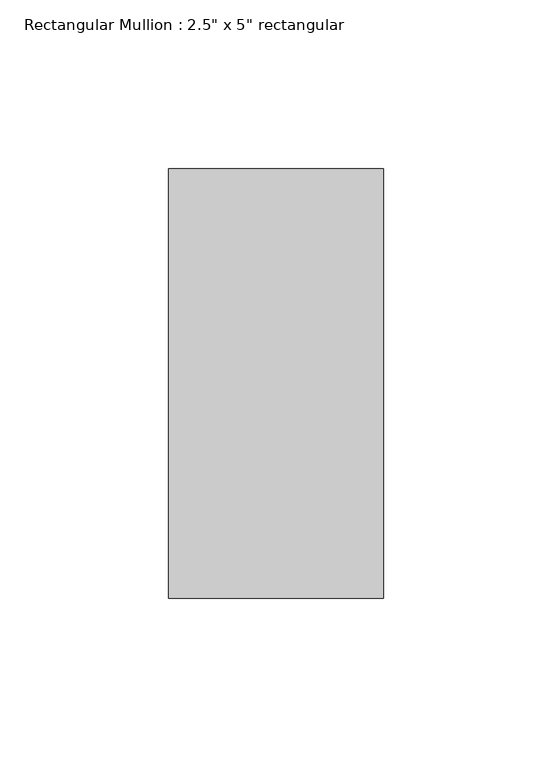
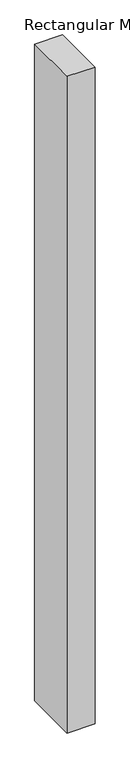
"""IFC4 building model written with IfcOpenShell, lengths in millimetres: member geometry."""

from ifc_helpers import new_model, si_unit, frame, origin, place, context, project, spatial, polyline, outline, extrude, source, transform, mapped, element, save


def member_acc0cca9(model_context):
    return source(origin(), model_context, "Body", "SweptSolid", [
        extrude(outline(polyline([(0.0, 63.5), (0.0, -63.5), (-63.5, -63.5), (-63.5, 63.5), (0.0, 63.5)])), frame((0.0, 0.0, -1570.4687519), z_axis=(0.0, 0.0, 1.0), x_axis=(1.0, 0.0, 0.0)), (0.0, 0.0, 1.0), 1570.4687519),
    ])


if __name__ == "__main__":
    model = new_model("IFC4")
    model_context = context("Model", 3, world=origin())
    ifc_project = project(units=[si_unit("LENGTHUNIT", "METRE", prefix="MILLI")], contexts=[model_context])
    site = spatial("IfcSite", under=ifc_project)
    building = spatial("IfcBuilding", under=site)
    placement = place(None, origin())
    member_shape = member_acc0cca9(model_context)
    element("IfcMember", 1, ObjectType="Rectangular Mullion : 2.5\" x 5\" rectangular", at=placement, inside=building, context=model_context, shape_type="MappedRepresentation", body=[
        mapped(member_shape, transform((0.0, 0.0, 0.0), x_axis=(1.0, 0.0, 0.0), y_axis=(0.0, 1.0, 0.0), z_axis=(0.0, 0.0, 1.0))),
    ])
    save(model, "model.ifc")

# Revit data of these elements
# Type "Rectangular Mullion : 2.5\" x 5\" rectangular"
#   built-in parameter 1007304 = 0.416667 (stored number, unit not read)
#   built-in parameter 1007301 = 0.104167 (stored number, unit not read)
#   built-in parameter 1007300 = 0.104167 (stored number, unit not read)
# Element 1 (IfcMember, "Rectangular Mullion : 2.5\" x 5\" rectangular")
#   Materials on its faces: "Aluminum"
# Materials
#   "Aluminum": class "Metal", colour RGB 247 247 247, transparency 0, Description = "Aluminum 6061", Cost = 0
